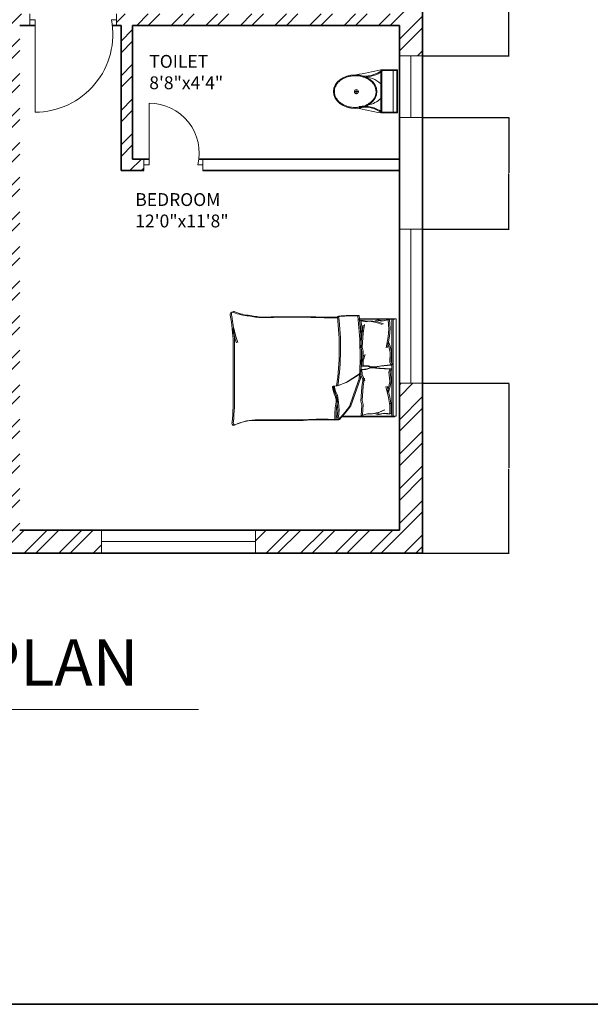
# Model space of a CAD drawing. Units: inches. Extents: x 1152 to 2588, y 1459 to 2618.
# Tile 3 of 17: x 1579 to 1802, y 1459 to 1843. Entities that reach past the tile are written whole.
import ezdxf

# ---------------------------------------------------------------- set-up
doc = ezdxf.new("R2010")
doc.units = ezdxf.units.IN
for name, color, linetype, lineweight in [('A-ANNO-DIMS', 2, 'Continuous', 18), ('A-ANNO-TEXT', 7, 'Continuous', 18), ('A-ANNO-TTLB', 7, 'Continuous', 35), ('A-AREA-IDEN', 7, 'Continuous', 18), ('A-DOOR', 4, 'Continuous', 18), ('A-FLOR-FIXT', 9, 'Continuous', 18), ('A-FURN', 8, 'Continuous', 13), ('A-GLAZ', 4, 'Continuous', 18), ('A-WALL', 7, 'Continuous', 35), ('A-WALL-PATT', 8, 'Continuous', 13)]:
    doc.layers.add(name, color=color, linetype=linetype, lineweight=lineweight)
doc.styles.get("Standard").update_dxf_attribs({"font": 'arial.ttf'})
doc.dimstyles.get("Standard").update_dxf_attribs({"dimtxt": 0.18, "dimasz": 0.18, "dimexe": 0.18, "dimexo": 0.0625, "dimgap": 0.09, "dimtad": 0, "dimtih": 1, "dimtoh": 1, "dimdec": 4, "dimzin": 0, "dimdsep": 46, "dimtxsty": 'Standard', "dimcen": 0.09, "dimadec": 0, "dimazin": 0, "dimtfac": 1, "dimtdec": 4, "dimtofl": 0, "dimtmove": 0, "dimatfit": 3, "dimfxl": 1, "dimtolj": 1, "dimtzin": 0, "dimarcsym": 0})

# ---------------------------------------------------------------- blocks, each defined once
blk = doc.blocks.new('A$C31115884')
for p, q in [((283, 498), (223, 498)), ((258, 466), (258, 523)), ((0, 200), (0, 0)), ((520, 200), (0, 200)), ((10, 190), (10, 10)), ((510, 190), (10, 190)), ((510, 10), (510, 190)), ((520, 0), (520, 200)), ((510, 54), (0, 54)), ((10, 10), (510, 10)), ((0, 0), (520, 0))]:
    blk.add_line(p, q)
blk.add_circle((256, 496), 23.6)
for centre, radius, start, end in [((2778, -205), 2807, 165.4549, 171.7133), ((3237, 905), 2807, 188.2867, 194.5451), ((-295, 403), 365, 324.2091, 9.3499), ((-295, 403), 375, 324.2091, 9.3499), ((139, 406), 293, 315.8436, 2.6563), ((806, 403), 375, 179.2036, 215.7909), ((806, 403), 365, 170.6501, 215.7909), ((384, 406), 293, 190.2774, 224.1564)]:
    blk.add_arc(centre, radius, start, end)
blk.add_ellipse((256, 510), major_axis=(0, -261), ratio=0.772727)
blk.add_open_spline([(256, 259), (263, 259), (270, 260), (288, 262), (299, 265), (320, 273), (330, 278), (350, 291), (360, 299), (378, 316), (386, 326), (402, 347), (409, 358), (421, 383), (427, 395), (436, 422), (440, 436), (445, 465), (447, 480), (448, 509), (448, 524), (445, 553), (443, 568), (436, 596), (432, 610), (422, 636), (416, 649), (402, 672), (395, 683), (379, 703), (370, 712), (351, 728), (341, 735), (321, 746), (310, 751), (289, 757), (278, 759), (256, 761), (245, 761), (223, 757), (212, 754), (191, 746), (181, 741), (161, 728), (151, 720), (133, 703), (125, 693), (110, 672), (103, 660), (90, 636), (85, 623), (76, 596), (72, 582), (67, 553), (66, 538), (64, 509), (65, 494), (68, 465), (70, 450), (77, 422), (81, 408), (91, 382), (97, 370), (111, 346), (118, 335), (135, 316), (144, 307), (162, 291), (172, 284), (193, 273), (203, 269), (225, 262), (236, 260), (250, 259), (253, 259), (256, 259)], degree=3, knots=[0, 0, 0, 0, 0.110105, 0.110105, 0.285049, 0.285049, 0.459994, 0.459994, 0.634938, 0.634938, 0.809882, 0.809882, 0.984827, 0.984827, 1.159771, 1.159771, 1.334715, 1.334715, 1.50966, 1.50966, 1.684604, 1.684604, 1.859549, 1.859549, 2.034493, 2.034493, 2.209437, 2.209437, 2.384382, 2.384382, 2.559326, 2.559326, 2.73427, 2.73427, 2.909215, 2.909215, 3.084159, 3.084159, 3.259103, 3.259103, 3.434048, 3.434048, 3.608992, 3.608992, 3.783936, 3.783936, 3.958881, 3.958881, 4.133825, 4.133825, 4.30877, 4.30877, 4.483714, 4.483714, 4.658658, 4.658658, 4.833603, 4.833603, 5.008547, 5.008547, 5.183491, 5.183491, 5.358436, 5.358436, 5.53338, 5.53338, 5.708324, 5.708324, 5.883269, 5.883269, 6.058213, 6.058213, 6.233158, 6.233158, 6.283185, 6.283185, 6.283185, 6.283185])
blk = doc.blocks.new('BED-PLAN')
for p, q in [((49.83, 41.36), (64.23, 41.36)), ((49.83, 41.36), (64.23, 41.36)), ((50.34, 41.54), (64.74, 41.54)), ((50.34, 41.54), (64.74, 41.54)), ((51.02, 36.75), (50.45, 40.8)), ((50.45, 40.8), (52.97, 40.34)), ((51.02, 36.75), (50.45, 40.8)), ((50.45, 40.8), (52.97, 40.34)), ((51.53, 36.93), (50.95, 40.98)), ((50.95, 40.98), (53.48, 40.52)), ((51.53, 36.93), (50.95, 40.98)), ((50.95, 40.98), (53.48, 40.52)), ((51.81, 39.05), (51.28, 35.85)), ((51.81, 39.05), (51.28, 35.85)), ((52.32, 39.23), (51.79, 36.03)), ((52.32, 39.23), (51.79, 36.03)), ((52.97, 40.34), (54.24, 40.57)), ((52.97, 40.34), (54.24, 40.57)), ((53.48, 40.52), (54.75, 40.75)), ((53.48, 40.52), (54.75, 40.75)), ((54.24, 40.57), (57.11, 40.11)), ((54.24, 40.57), (57.11, 40.11)), ((54.75, 40.75), (57.62, 40.29)), ((54.75, 40.75), (57.62, 40.29)), ((57, 40.91), (56.19, 40.45)), ((57, 40.91), (56.19, 40.45)), ((57.51, 41.09), (56.7, 40.64)), ((57.51, 41.09), (56.7, 40.64)), ((59.07, 40.57), (57, 40.91)), ((59.07, 40.57), (57, 40.91)), ((57.11, 40.11), (59.3, 39.3)), ((57.11, 40.11), (59.3, 39.3)), ((59.57, 40.75), (57.51, 41.09)), ((59.57, 40.75), (57.51, 41.09)), ((57.62, 40.29), (59.8, 39.49)), ((57.62, 40.29), (59.8, 39.49)), ((61.59, 41.03), (59.07, 40.57)), ((61.59, 41.03), (59.07, 40.57)), ((62.1, 41.21), (59.57, 40.75)), ((62.1, 41.21), (59.57, 40.75)), ((61.58, 41.03), (61.84, 37.62)), ((61.58, 41.02), (61.84, 37.62)), ((62.08, 41.21), (62.35, 37.8)), ((62.08, 41.21), (62.35, 37.8)), ((63.01, 41.36), (63.01, 3.37)), ((63.01, 41.36), (63.01, 3.37)), ((63.52, 41.54), (63.52, 3.56)), ((63.52, 41.54), (63.52, 3.56)), ((64.74, 41.54), (64.74, 3.56)), ((51.28, 35.85), (50.93, 30.27)), ((51.28, 35.85), (50.93, 30.27)), ((51.28, 35.85), (51.02, 36.75)), ((51.28, 35.85), (51.02, 36.75)), ((51.79, 36.03), (51.44, 30.46)), ((51.79, 36.03), (51.44, 30.46)), ((51.79, 36.03), (51.53, 36.93)), ((51.79, 36.03), (51.53, 36.93)), ((62.1, 34.68), (61.3, 30.31)), ((62.1, 34.68), (61.3, 30.31)), ((61.82, 37.54), (61.59, 34.5)), ((61.82, 37.54), (61.59, 34.5)), ((61.84, 37.62), (61.82, 37.54)), ((61.84, 37.62), (61.82, 37.54)), ((62.33, 37.72), (62.1, 34.68)), ((62.33, 37.72), (62.1, 34.68)), ((62.35, 37.8), (62.33, 37.72)), ((62.35, 37.8), (62.33, 37.72)), ((1.24, 32.15), (1.24, 12.59)), ((1.24, 32.15), (1.24, 12.59)), ((1.75, 32.33), (1.75, 12.77)), ((1.75, 32.33), (1.75, 12.77)), ((61.59, 34.5), (60.79, 30.13)), ((61.59, 34.5), (60.79, 30.13)), ((61.25, 32.32), (61.82, 30.71)), ((61.25, 32.32), (61.82, 30.71)), ((61.76, 32.5), (62.33, 30.89)), ((61.76, 32.5), (62.33, 30.89)), ((61.82, 30.71), (62.4, 28.41)), ((61.82, 30.71), (62.4, 28.41)), ((62.33, 30.89), (62.91, 28.59)), ((62.33, 30.89), (62.91, 28.59)), ((50.93, 30.27), (51.38, 28.72)), ((50.93, 30.27), (51.38, 28.72)), ((51.38, 28.72), (51.06, 24.64)), ((51.38, 28.72), (51.06, 24.64)), ((51.3, 24.96), (52.17, 27.46)), ((51.3, 24.96), (52.17, 27.46)), ((51.44, 30.46), (51.89, 28.9)), ((51.44, 30.46), (51.89, 28.9)), ((51.89, 28.9), (51.56, 24.82)), ((51.89, 28.9), (51.56, 24.82)), ((51.81, 25.15), (52.68, 27.65)), ((51.81, 25.15), (52.68, 27.65)), ((62.4, 28.15), (62.28, 24.62)), ((62.4, 28.15), (62.28, 24.62)), ((62.4, 28.41), (62.4, 28.15)), ((62.4, 28.41), (62.4, 28.15)), ((62.91, 28.34), (62.79, 24.8)), ((62.91, 28.34), (62.79, 24.8)), ((62.91, 28.59), (62.91, 28.34)), ((62.91, 28.59), (62.91, 28.34)), ((51.3, 23.01), (51.3, 24.96)), ((51.3, 23.01), (51.3, 24.96)), ((53.43, 23.01), (51.3, 23.01)), ((53.43, 23.01), (51.3, 23.01)), ((51.81, 23.19), (51.81, 25.15)), ((51.81, 23.19), (51.81, 25.15)), ((53.94, 23.19), (51.81, 23.19)), ((53.94, 23.19), (51.81, 23.19)), ((54.93, 22.55), (53.43, 23.01)), ((54.93, 22.55), (53.43, 23.01)), ((55.44, 22.73), (53.94, 23.19)), ((55.44, 22.73), (53.94, 23.19)), ((58.49, 23.01), (55.96, 22.55)), ((58.49, 23.01), (55.96, 22.55)), ((59, 23.19), (56.47, 22.73)), ((59, 23.19), (56.47, 22.73)), ((62.74, 23.47), (58.49, 23.01)), ((62.74, 23.47), (58.49, 23.01)), ((63.25, 23.65), (59, 23.19)), ((63.25, 23.65), (59, 23.19)), ((62.28, 24.62), (62.74, 23.47)), ((62.28, 24.62), (62.74, 23.47)), ((62.79, 24.8), (63.25, 23.65)), ((62.79, 24.8), (63.25, 23.65)), ((50.41, 20.07), (45.25, 16.74)), ((50.41, 20.07), (45.25, 16.74)), ((50.92, 20.25), (45.76, 16.92)), ((50.92, 20.25), (45.76, 16.92)), ((52.93, 21.76), (50.8, 21.63)), ((52.93, 21.76), (50.8, 21.63)), ((50.8, 21.63), (50.92, 19.68)), ((50.8, 21.63), (50.92, 19.68)), ((50.92, 19.68), (51.95, 17.24)), ((50.92, 19.68), (51.95, 17.24)), ((53.44, 21.95), (51.31, 21.81)), ((53.44, 21.94), (51.31, 21.81)), ((51.31, 21.81), (51.43, 19.86)), ((51.31, 21.81), (51.43, 19.86)), ((51.43, 19.86), (52.45, 17.42)), ((51.43, 19.86), (52.45, 17.42)), ((54.39, 22.32), (52.93, 21.76)), ((54.39, 22.32), (52.93, 21.76)), ((54.9, 22.5), (53.44, 21.94)), ((54.9, 22.5), (53.44, 21.95)), ((55.42, 22.38), (54.39, 22.32)), ((55.42, 22.38), (54.39, 22.32)), ((55.93, 22.56), (54.9, 22.5)), ((55.93, 22.56), (54.9, 22.5)), ((55.96, 22.55), (54.93, 22.55)), ((55.96, 22.55), (54.93, 22.55)), ((57.98, 22.08), (55.42, 22.38)), ((57.98, 22.08), (55.42, 22.38)), ((56.47, 22.73), (55.44, 22.73)), ((56.47, 22.73), (55.44, 22.73)), ((58.48, 22.26), (55.93, 22.56)), ((58.48, 22.26), (55.93, 22.56)), ((62.25, 21.89), (57.98, 22.08)), ((62.25, 21.89), (57.98, 22.08)), ((62.76, 22.07), (58.48, 22.26)), ((62.76, 22.07), (58.48, 22.26)), ((61.86, 20.71), (62.25, 21.89)), ((61.86, 20.71), (62.25, 21.89)), ((62.2, 17.19), (61.86, 20.71)), ((62.2, 17.19), (61.86, 20.71)), ((62.37, 20.89), (62.76, 22.07)), ((62.37, 20.89), (62.76, 22.07)), ((62.71, 17.37), (62.37, 20.89)), ((62.71, 17.37), (62.37, 20.89)), ((41.68, 15.39), (40.08, 15.14)), ((41.68, 15.39), (40.08, 15.14)), ((42.19, 15.57), (40.59, 15.32)), ((42.19, 15.57), (40.59, 15.32)), ((45.25, 16.74), (41.68, 15.39)), ((45.25, 16.74), (41.68, 15.39)), ((45.76, 16.92), (42.19, 15.57)), ((45.76, 16.92), (42.19, 15.57)), ((48.08, 11.82), (50.41, 18.44)), ((48.08, 11.82), (50.41, 18.44)), ((48.59, 12), (50.92, 18.63)), ((48.59, 12), (50.92, 18.63)), ((51.81, 18.24), (51.28, 15.03)), ((51.81, 18.24), (51.28, 15.03)), ((52.32, 18.42), (51.79, 15.22)), ((52.32, 18.42), (51.79, 15.22)), ((61.78, 14.61), (62.21, 16.94)), ((61.78, 14.61), (62.21, 16.94)), ((62.21, 16.94), (62.2, 17.19)), ((62.21, 16.94), (62.2, 17.19)), ((62.29, 14.79), (62.72, 17.12)), ((62.29, 14.79), (62.72, 17.12)), ((62.72, 17.12), (62.71, 17.37)), ((62.72, 17.12), (62.71, 17.37)), ((40.08, 15.14), (40.58, 13.17)), ((40.08, 15.14), (40.58, 13.17)), ((40.58, 13.17), (41.31, 11.57)), ((40.58, 13.17), (41.31, 11.57)), ((40.59, 15.32), (41.08, 13.35)), ((40.59, 15.32), (41.08, 13.35)), ((41.08, 13.35), (41.82, 11.75)), ((41.08, 13.35), (41.82, 11.75)), ((41.31, 11.57), (41.68, 8.86)), ((41.31, 11.57), (41.68, 8.86)), ((41.82, 11.75), (42.19, 9.04)), ((41.82, 11.75), (42.19, 9.04)), ((46.48, 7.38), (48.08, 11.82)), ((46.48, 7.38), (48.08, 11.82)), ((46.99, 7.57), (48.59, 12)), ((46.99, 7.57), (48.59, 12)), ((51.28, 15.03), (50.93, 9.46)), ((51.28, 15.03), (50.93, 9.46)), ((51.79, 15.22), (51.44, 9.64)), ((51.79, 15.22), (51.44, 9.64)), ((61.79, 10.81), (60.71, 15.11)), ((61.79, 10.81), (60.71, 15.11)), ((62.3, 10.99), (61.22, 15.3)), ((62.3, 10.99), (61.22, 15.3)), ((61.31, 12.96), (61.78, 14.61)), ((61.31, 12.96), (61.78, 14.61)), ((61.82, 13.15), (62.29, 14.79)), ((61.82, 13.15), (62.29, 14.79)), ((41.68, 8.86), (41.93, 5.78)), ((41.68, 8.86), (41.93, 5.78)), ((42.19, 9.04), (42.44, 5.97)), ((42.19, 9.04), (42.44, 5.97)), ((50.93, 9.46), (51.38, 7.9)), ((50.93, 9.46), (51.38, 7.9)), ((51.38, 7.9), (51.06, 3.82)), ((51.38, 7.9), (51.06, 3.82)), ((51.44, 9.64), (51.89, 8.09)), ((51.44, 9.64), (51.89, 8.09)), ((51.89, 8.09), (51.56, 4.01)), ((51.89, 8.09), (51.56, 4.01)), ((62.21, 7.79), (61.79, 10.81)), ((62.21, 7.79), (61.79, 10.81)), ((62.2, 4.29), (62.27, 8.59)), ((62.2, 4.29), (62.27, 8.58)), ((62.27, 8.59), (62.21, 7.79)), ((62.27, 8.58), (62.21, 7.79)), ((62.72, 7.97), (62.3, 10.99)), ((62.72, 7.97), (62.3, 10.99)), ((62.71, 4.47), (62.78, 8.77)), ((62.71, 4.47), (62.78, 8.77)), ((62.78, 8.77), (62.72, 7.97)), ((62.78, 8.77), (62.72, 7.97)), ((41.93, 5.78), (41.68, 3.32)), ((41.93, 5.78), (41.68, 3.32)), ((42.18, 2.1), (44.76, 5.05)), ((42.18, 2.1), (44.76, 5.05)), ((42.44, 5.97), (42.19, 3.5)), ((42.44, 5.97), (42.19, 3.5)), ((42.68, 2.28), (45.27, 5.23)), ((42.68, 2.28), (45.27, 5.23)), ((44.76, 5.05), (46.48, 7.38)), ((44.76, 5.05), (46.48, 7.38)), ((45.27, 5.23), (46.99, 7.57)), ((45.27, 5.23), (46.99, 7.57)), ((51.06, 3.82), (53.55, 4.44)), ((51.06, 3.82), (53.55, 4.44)), ((51.56, 4.01), (54.06, 4.62)), ((51.56, 4.01), (54.06, 4.62)), ((53.55, 4.44), (54.83, 4.29)), ((53.55, 4.44), (54.83, 4.29)), ((54.06, 4.62), (55.34, 4.47)), ((54.06, 4.62), (55.34, 4.47)), ((54.83, 4.29), (57.67, 4.93)), ((54.83, 4.29), (57.67, 4.93)), ((55.34, 4.47), (58.17, 5.11)), ((55.34, 4.47), (58.17, 5.11)), ((57.6, 4.12), (56.77, 4.53)), ((57.6, 4.12), (56.77, 4.53)), ((58.11, 4.3), (57.28, 4.71)), ((58.11, 4.3), (57.28, 4.71)), ((59.65, 4.59), (57.6, 4.12)), ((59.65, 4.59), (57.6, 4.12)), ((57.67, 4.93), (59.8, 5.87)), ((57.67, 4.93), (59.8, 5.87)), ((60.15, 4.77), (58.11, 4.3)), ((60.15, 4.77), (58.11, 4.3)), ((58.17, 5.11), (60.3, 6.05)), ((58.17, 5.11), (60.3, 6.05)), ((62.2, 4.29), (59.65, 4.59)), ((62.2, 4.29), (59.65, 4.59)), ((62.71, 4.47), (60.15, 4.77)), ((62.71, 4.47), (60.15, 4.77)), ((40.79, 2.04), (42.18, 2.1, 3.08)), ((40.79, 2.04), (42.18, 2.1, 3.08)), ((41.3, 2.22), (42.68, 2.28, 3.08)), ((41.3, 2.22), (42.68, 2.28, 3.08)), ((41.68, 3.32), (42.18, 2.1)), ((41.68, 3.32), (42.18, 2.1)), ((42.19, 3.5), (42.68, 2.28)), ((42.19, 3.5), (42.68, 2.28)), ((64.23, 3.37), (43.08, 3.37)), ((64.23, 3.37), (43.08, 3.37)), ((64.74, 3.56), (43.59, 3.56)), ((64.74, 3.56), (43.59, 3.56))]:
    blk.add_line(p, q)
for centre, radius, start, end in [((0.86, 43.26), 0.866, 56.1736, 203.4781), ((0.86, 43.26), 0.866, 56.1736, 203.4781), ((-95.41, 27.09), 96.78, 2.9958, 9.4091), ((-95.41, 27.09), 96.78, 2.9958, 9.4091), ((1.37, 43.44), 0.866, 56.1736, 203.4781), ((1.37, 43.44), 0.866, 56.1736, 203.4781), ((-94.9, 27.27), 96.78, 2.9958, 9.4091), ((-94.9, 27.27), 96.78, 2.9958, 9.4091), ((8.37, 61.34), 18.73, 247.9751, 266.652), ((8.37, 61.34), 18.73, 247.9751, 266.652), ((8.88, 61.52), 18.73, 247.9751, 266.652), ((8.88, 61.52), 18.73, 247.9751, 266.652), ((12.95, 65.51), 23.56, 256.0648, 268.9113), ((12.95, 65.51), 23.56, 256.0648, 268.9113), ((13.46, 65.69), 23.56, 256.0648, 268.9113), ((13.46, 65.69), 23.56, 256.0648, 268.9113), ((24.51, -341.07), 383.38, 88.2277, 91.7185), ((24.51, -341.07), 383.38, 88.2277, 91.7185), ((-60.02, 30.01), 102.56, 351.7845, 6.9006), ((-60.02, 30.01), 102.56, 351.7845, 6.9006), ((48.26, -23.57), 66.22, 88.7218, 95.604), ((48.26, -23.57), 66.22, 88.7218, 95.604), ((-59.52, 30.19), 102.56, 351.7845, 6.9006), ((-59.52, 30.19), 102.56, 351.7845, 6.9006), ((48.76, -23.39), 66.22, 88.7218, 95.604), ((48.76, -23.39), 66.22, 88.7218, 95.604), ((-80.48, 27.15), 131.13, 356.0865, 6.7821), ((-80.48, 27.15), 131.13, 356.0865, 6.7821), ((-79.97, 27.33), 131.13, 356.0865, 6.7821), ((-79.97, 27.33), 131.13, 356.0865, 6.7821), ((83.59, 57.99), 84.62, 193.3832, 197.7053), ((83.59, 57.99), 84.62, 193.3832, 197.7053), ((24, -341.25), 383.38, 88.2277, 91.7185), ((24, -341.25), 383.38, 88.2277, 91.7185), ((39.45, 177.11), 135.22, 268.4762, 271.0082), ((39.45, 177.11), 135.22, 268.4762, 271.0082), ((39.96, 177.3), 135.22, 268.4762, 271.0082), ((39.96, 177.3), 135.22, 268.4762, 271.0082), ((83.08, 57.81), 84.62, 193.3832, 197.7053), ((83.08, 57.81), 84.62, 193.3832, 197.7053), ((-104.51, 11.41), 105.75, 354.4998, 0.6351), ((-104.51, 11.41), 105.75, 354.4998, 0.6351), ((-104, 11.59), 105.75, 354.4998, 0.6351), ((-104, 11.59), 105.75, 354.4998, 0.6351), ((40.03, 15), 0.147, 70.2464, 181.1377), ((40.03, 15), 0.147, 70.2464, 181.1377), ((63.05, 19.36), 23.57, 190.6617, 199.8806), ((63.05, 19.36), 23.57, 190.6617, 199.8806), ((40.54, 15.18), 0.147, 70.2464, 181.1377), ((40.54, 15.18), 0.147, 70.2464, 181.1377), ((63.56, 19.54), 23.57, 190.6617, 199.8806), ((63.56, 19.54), 23.57, 190.6617, 199.8806), ((36.86, 9.53), 4.95, 348.6608, 23.7384), ((36.86, 9.53), 4.95, 348.6608, 23.7384), ((69.52, 3.32), 28.76, 169.8763, 182.5657), ((69.52, 3.32), 28.76, 169.8763, 182.5657), ((36.36, 9.35), 4.95, 348.6608, 23.7384), ((36.36, 9.35), 4.95, 348.6608, 23.7384), ((70.03, 3.51), 28.76, 169.8763, 182.5657), ((70.03, 3.51), 28.76, 169.8763, 182.5657), ((1.54, 0.87), 0.876, 152.6588, 266.02), ((1.54, 0.87), 0.876, 152.6588, 266.02), ((2.05, 1.06), 0.876, 152.6588, 266.02), ((2.05, 1.06), 0.876, 152.6588, 266.02), ((9.65, -16.41), 18.33, 87.4714, 116.4681), ((9.65, -16.41), 18.33, 87.4714, 116.4681), ((10.16, -16.23), 18.33, 87.4714, 116.4681), ((10.16, -16.23), 18.33, 87.4714, 116.4681), ((10.32, 3628.06), 3626.16, 270.00217, 270.28689), ((10.32, 3628.06), 3626.16, 270.00217, 270.28689), ((10.83, 3628.24), 3626.16, 270.00217, 270.28689), ((10.83, 3628.24), 3626.16, 270.00217, 270.28689), ((35.36, -100.76), 102.94, 86.9791, 93.8365), ((35.36, -100.76), 102.94, 86.9791, 93.8365), ((35.87, -100.58), 102.94, 86.9791, 93.8365), ((35.87, -100.57), 102.94, 86.9791, 93.8365)]:
    blk.add_arc(centre, radius, start, end)
blk = doc.blocks.new('DOOR-24-ENSUITE')
for p, q in [((2, 2.25), (2, 26.25)), ((0, 4.5), (0, 0)), ((23, 4.5), (23, 0)), ((0, 2.25), (2, 2.25)), ((23, 2.25), (21, 2.25)), ((23, 0), (23, 2.25)), ((23, 2.25), (23, 2.25)), ((0, 0), (0, 0))]:
    blk.add_line(p, q)
blk.add_arc((2, 6.73), 19.52, 346.721, 90)
blk = doc.blocks.new('DOOR-36-HALL')
for p, q in [((0, 33.75), (0, 38.25)), ((0, 38.25), (0, 36)), ((0, 36), (2, 36)), ((2, 36), (2, 0)), ((33.77, 36), (31.77, 36)), ((33.77, 33.75), (33.77, 38.25)), ((33.77, 38.25), (33.77, 36))]:
    blk.add_line(p, q)
blk.add_arc((2, 30.31), 30.31, 270, 10.8162)
blk = doc.blocks.new('WIN-60-EXT')
for p, q in [((0, 9), (0, 0)), ((60, 4.5), (60, 9)), ((60, 9), (60, 0)), ((0, 0), (0, 4.5)), ((0, 4.5), (60, 4.5))]:
    blk.add_line(p, q)
blk = doc.blocks.new('WIN-24-BATH-EAST')
for p, q in [((0, 24), (9, 24)), ((9, 24), (4.5, 24)), ((4.5, 24), (4.5, 0)), ((4.5, 0), (0, 0)), ((0, 0), (9, 0))]:
    blk.add_line(p, q)
blk = doc.blocks.new('*D72')
at = {"layer": 'A-ANNO-DIMS', "color": 0, "lineweight": -2, "transparency": 16777216}
for p, q in [((1736.48, 1701.19), (1770.2, 1701.19)), ((1770.02, 1701.01), (1770.02, 1668.3)), ((1770.02, 1635.23), (1770.02, 1667.93)), ((1736.48, 1635.05), (1770.2, 1635.05))]:
    blk.add_line(p, q, dxfattribs=at)
at = {"layer": 'A-ANNO-DIMS', "color": 0, "transparency": 16777216}
for points in [[(1769.99, 1701.01), (1770.05, 1701.01), (1770.02, 1701.19)], [(1769.99, 1635.23), (1770.05, 1635.23), (1770.02, 1635.05)]]:
    blk.add_solid(points, dxfattribs=at)
at = {"layer": 'Defpoints', "color": 0, "transparency": 16777216}
for p in [(1736.42, 1701.19), (1770.02, 1701.19), (1736.42, 1635.05)]:
    blk.add_point(p, dxfattribs=at)
at = {"layer": 'A-ANNO-DIMS', "color": 0, "transparency": 16777216, "insert": (1770.02, 1668.12), "char_height": 0.18, "attachment_point": 5}
blk.add_mtext('\\A1;66.14', dxfattribs=at)
blk = doc.blocks.new('*D73')
at = {"layer": 'A-ANNO-DIMS', "color": 0, "lineweight": -2, "transparency": 16777216}
for p, q in [((1736.48, 1804.76), (1770.2, 1804.76)), ((1770.02, 1804.58), (1770.02, 1783.16)), ((1770.02, 1761.37), (1770.02, 1782.79)), ((1736.48, 1761.19), (1770.2, 1761.19))]:
    blk.add_line(p, q, dxfattribs=at)
at = {"layer": 'A-ANNO-DIMS', "color": 0, "transparency": 16777216}
for points in [[(1769.99, 1804.58), (1770.05, 1804.58), (1770.02, 1804.76)], [(1769.99, 1761.37), (1770.05, 1761.37), (1770.02, 1761.19)]]:
    blk.add_solid(points, dxfattribs=at)
at = {"layer": 'Defpoints', "color": 0, "transparency": 16777216}
for p in [(1736.42, 1804.76), (1770.02, 1804.76), (1736.42, 1761.19)]:
    blk.add_point(p, dxfattribs=at)
at = {"layer": 'A-ANNO-DIMS', "color": 0, "transparency": 16777216, "insert": (1770.02, 1782.97), "char_height": 0.18, "attachment_point": 5}
blk.add_mtext('\\A1;43.576', dxfattribs=at)
blk = doc.blocks.new('*D74')
at = {"layer": 'A-ANNO-DIMS', "color": 0, "lineweight": -2, "transparency": 16777216}
for p, q in [((1736.48, 1875.36), (1770.2, 1875.36)), ((1770.02, 1875.18), (1770.02, 1852.24)), ((1770.02, 1828.94), (1770.02, 1851.88)), ((1736.48, 1828.76), (1770.2, 1828.76))]:
    blk.add_line(p, q, dxfattribs=at)
at = {"layer": 'A-ANNO-DIMS', "color": 0, "transparency": 16777216}
for points in [[(1769.99, 1875.18), (1770.05, 1875.18), (1770.02, 1875.36)], [(1769.99, 1828.94), (1770.05, 1828.94), (1770.02, 1828.76)]]:
    blk.add_solid(points, dxfattribs=at)
at = {"layer": 'Defpoints', "color": 0, "transparency": 16777216}
for p in [(1736.42, 1875.36), (1770.02, 1875.36), (1736.42, 1828.76)]:
    blk.add_point(p, dxfattribs=at)
at = {"layer": 'A-ANNO-DIMS', "color": 0, "transparency": 16777216, "insert": (1770.02, 1852.06), "char_height": 0.18, "attachment_point": 5}
blk.add_mtext('\\A1;46.59', dxfattribs=at)

msp = doc.modelspace()

# ---------------------------------------------------------------- hatches: boundary and pattern name
at = {"layer": 'A-WALL-PATT'}
h = msp.add_hatch(dxfattribs=at)
h.set_pattern_fill('ANSI32', color=256)
h.paths.add_polyline_path([(1408.9272, 2240.0458), (1276.4165, 2240.0458), (1276.4165, 2192.7491), (1285.4165, 2192.7491), (1285.4165, 2231.0458), (1369.4165, 2231.0458), (1369.4165, 2084.0458), (1526.9165, 2084.0458), (1526.9165, 2096.3728), (1524.6665, 2096.3728), (1522.4165, 2096.3728), (1522.4165, 2093.0458), (1378.4165, 2093.0458), (1378.4165, 2231.0458), (1408.9272, 2231.0458)])
h.paths.add_polyline_path([(1736.4165, 2240.0458), (1468.9272, 2240.0458), (1468.9272, 2231.0458), (1522.4165, 2231.0458), (1522.4165, 2127.3313), (1526.9165, 2127.3313), (1526.9165, 2231.0458), (1574.9165, 2231.0458), (1574.9165, 2188.0458), (1579.4165, 2188.0458), (1579.4165, 2231.0458), (1727.4165, 2231.0458), (1727.4165, 2183.9728), (1736.4165, 2183.9728)])
h.paths.add_polyline_path([(1285.4165, 2156.7491), (1276.4165, 2156.7491), (1276.4165, 2084.0458), (1285.4165, 2084.0458)], flags=17)
h.paths.add_polyline_path([(1285.4165, 2043.5458), (1445.4165, 2043.5458), (1445.4165, 1943.6503), (1454.4165, 1943.6503), (1454.4165, 2048.0458), (1276.4165, 2048.0458), (1276.4165, 2019.2077), (1280.9165, 2019.2077), (1285.4165, 2019.2077)])
h.paths.add_polyline_path([(1285.4165, 1959.2077), (1276.4165, 1959.2077), (1276.4165, 1891.1319), (1280.9165, 1891.1319), (1285.4165, 1891.1319), (1285.4165, 1901.0458), (1376.8505, 1901.0458), (1376.8505, 1903.2958), (1376.8505, 1905.5458), (1285.4165, 1905.5458)])
h.paths.add_polyline_path([(1518.4165, 1905.5458), (1399.2832, 1905.5458), (1399.2832, 1903.2958), (1399.2832, 1901.0458), (1405.4165, 1901.0458), (1405.4165, 1884.8579), (1409.9165, 1884.8579), (1409.9165, 1901.0458), (1513.9165, 1901.0458), (1513.9165, 1869.1706), (1518.4165, 1869.1706)])
h.paths.add_polyline_path([(1520.5229, 1845.0458), (1518.4165, 1845.0458), (1518.4165, 1849.2927), (1516.1665, 1849.2927), (1513.9165, 1849.2927), (1513.9165, 1845.0458), (1409.9165, 1845.0458), (1409.9165, 1860.8579), (1405.4165, 1860.8579), (1405.4165, 1845.0458), (1285.4165, 1845.0458), (1285.4165, 1867.1319), (1276.4165, 1867.1319), (1276.4165, 1635.0458), (1285.4165, 1635.0458), (1285.4165, 1836.0458), (1405.4165, 1836.0458), (1405.4165, 1635.0458), (1414.4165, 1635.0458), (1424.7277, 1635.0458), (1424.7277, 1639.5458), (1424.7277, 1644.0458), (1414.4165, 1644.0458), (1414.4165, 1836.0458), (1414.4165, 1840.5831), (1520.5229, 1840.5831)])
h.paths.add_polyline_path([(1579.4165, 1840.5458), (1583.4035, 1840.5458), (1583.4035, 1845.0458), (1579.4165, 1845.0458), (1570.4165, 1845.0458), (1570.4165, 1840.5831), (1570.4165, 1644.0458), (1548.2359, 1644.0458), (1548.2359, 1635.0458), (1611.2801, 1635.0458), (1611.2801, 1639.5458), (1611.2801, 1644.0458), (1579.4165, 1644.0458)])
h.paths.add_polyline_path([(1488.2359, 1644.0458), (1472.0663, 1644.0458), (1472.0663, 1635.0458), (1488.2359, 1635.0458), (1488.2359, 1639.5458)], flags=17)
h.paths.add_polyline_path([(1736.4165, 1701.1863), (1727.4165, 1701.1863), (1727.4165, 1644.0458), (1671.2801, 1644.0458), (1671.2801, 1635.0458), (1736.4165, 1635.0458)])
h.paths.add_polyline_path([(1736.4165, 2147.9728), (1727.4165, 2147.9728), (1727.4165, 2093.0458), (1579.4165, 2093.0458), (1574.9165, 2093.0458), (1574.9165, 1971.6501), (1579.4165, 1971.6501), (1579.4165, 2084.0458), (1727.4165, 2084.0458), (1727.4165, 2054.3847), (1736.4165, 2054.3847)])
h.paths.add_polyline_path([(1736.4165, 1994.3847), (1727.4165, 1994.3847), (1727.4165, 1911.3562), (1736.4165, 1911.3562)])
h.paths.add_polyline_path([(1736.4165, 1875.3562), (1727.4165, 1875.3562), (1727.4165, 1845.0458), (1617.1767, 1845.0458), (1617.1767, 1842.7958), (1617.1767, 1840.5458), (1618.9165, 1840.5458), (1618.9165, 1788.5458), (1618.9165, 1784.0458), (1627.8699, 1784.0458), (1627.8699, 1788.5458), (1623.4165, 1788.5458), (1623.4165, 1840.5458), (1727.4165, 1840.5458), (1727.4165, 1828.7619), (1736.4165, 1828.7619)])
h.paths.add_polyline_path([(1727.4165, 1938.0458), (1579.4165, 1938.0458), (1579.4165, 1942.7722), (1574.9165, 1942.7722), (1574.9165, 1929.0458), (1727.4165, 1929.0458)])

# ---------------------------------------------------------------- linework, layer by layer
at = {"layer": 'A-ANNO-TEXT'}
msp.add_line((1370.1295, 1574.1335), (1649.1589, 1574.1335), dxfattribs=at)
at = {"layer": 'A-ANNO-TTLB'}
msp.add_lwpolyline([(1152.3215, 2617.6685), (2587.6987, 2617.6685), (2587.6987, 1459.3148), (1152.3215, 1459.3148)], close=True, dxfattribs=at)
at = {"layer": 'A-WALL'}
for p, q in [((1736.4165, 2240.0458), (1736.4165, 1635.0458)), ((1579.4165, 1840.5458), (1585.4035, 1840.5458)), ((1615.5196, 1840.5458), (1618.9165, 1840.5458)), ((1618.9165, 1840.5458), (1618.9165, 1788.5458)), ((1623.4165, 1788.5458), (1623.4165, 1840.5458)), ((1623.4165, 1840.5458), (1727.4165, 1840.5458)), ((1727.4165, 1840.5458), (1727.4165, 1644.0458)), ((1727.4165, 1840.5458), (1727.4165, 1788.5458)), ((1618.9165, 1788.5458), (1618.9165, 1784.0458)), ((1629.8699, 1788.5458), (1623.4165, 1788.5458)), ((1727.4165, 1788.5458), (1649.2588, 1788.5458)), ((1618.9165, 1784.0458), (1627.8699, 1784.0458)), ((1650.8652, 1784.0458), (1727.4165, 1784.0458)), ((1579.4165, 1644.0458), (1727.4165, 1644.0458)), ((1472.0663, 1635.0458), (1736.4165, 1635.0458))]:
    msp.add_line(p, q, dxfattribs=at)

# ---------------------------------------------------------------- block references
at = {"layer": 'A-DOOR'}
for name, p in [('DOOR-36-HALL', (1583.404, 1806.796)), ('DOOR-24-ENSUITE', (1627.87, 1784.046))]:
    msp.add_blockref(name, p, dxfattribs=at)
at = {"layer": 'A-FLOR-FIXT', "xscale": 0.0323450304620732, "yscale": 0.0323450304620732, "zscale": 0.0323450304620732, "rotation": 89.99999999999999}
msp.add_blockref('A$C31115884', (1726.6942, 1806.5296), dxfattribs=at)
at = {"layer": 'A-FURN'}
msp.add_blockref('BED-PLAN', (1661.448, 1684.819), dxfattribs=at)
at = {"layer": 'A-GLAZ'}
for name, p in [('WIN-24-BATH-EAST', (1727.417, 1804.762)), ('WIN-60-EXT', (1611.28, 1635.046))]:
    msp.add_blockref(name, p, dxfattribs=at)
at = {"layer": 'A-GLAZ', "extrusion": (0, 0, -1), "zscale": -1, "rotation": 90}
msp.add_blockref('WIN-60-EXT', (-1727.4167, 1701.1862), dxfattribs=at)

# ---------------------------------------------------------------- texts
at = {"layer": 'A-ANNO-TEXT', "insert": (1371.0423, 1601.4677), "char_height": 18, "attachment_point": 1}
msp.add_mtext_dynamic_manual_height_columns('GROUND FLOOR PLAN ', width=297.615305, gutter_width=12.5, heights=[0], dxfattribs=at)
at = {"layer": 'A-AREA-IDEN', "char_height": 5, "attachment_point": 1}
for s, width, insert in [('TOILET\\P8\'8"x4\'4"', 104.234238, (1629.9323, 1829.0794)), ('BEDROOM\\P12\'0"x11\'8"', 114.677893, (1624.475, 1775.2541))]:
    msp.add_mtext_dynamic_manual_height_columns(s, width=width, gutter_width=12.5, heights=[0], dxfattribs=dict(at, insert=insert))

# ---------------------------------------------------------------- dimensions: what is measured, and where the dimension line sits
at = {"layer": 'A-ANNO-DIMS'}
for base, p1, p2, override, picture, middle in [((1770.0165, 1875.3562), (1736.4165, 1828.7619), (1736.4165, 1875.3562), {"dimdec": 2, "dimlfac": 1, "dimrnd": 0, "dimzin": 0, "dimdsep": 46, "dimlunit": 2}, '*D74', (1770.0165, 1852.0591)), ((1770.0165, 1804.7619), (1736.4165, 1761.1863), (1736.4165, 1804.7619), {"dimdec": 3, "dimlfac": 1, "dimrnd": 0, "dimzin": 0, "dimdsep": 46, "dimlunit": 2}, '*D73', (1770.0165, 1782.9741)), ((1770.0165, 1701.1863), (1736.4165, 1635.0458), (1736.4165, 1701.1863), {"dimdec": 2, "dimlfac": 1, "dimrnd": 0, "dimzin": 0, "dimdsep": 46, "dimlunit": 2}, '*D72', (1770.0165, 1668.1161))]:
    dim = msp.add_linear_dim(base=base, p1=p1, p2=p2, angle=90, dimstyle='Standard', override=override, dxfattribs=at)
    dim.commit()
    dim.dimension.update_dxf_attribs({"geometry": picture, "text_midpoint": middle})

doc.saveas('drawing.dxf')
